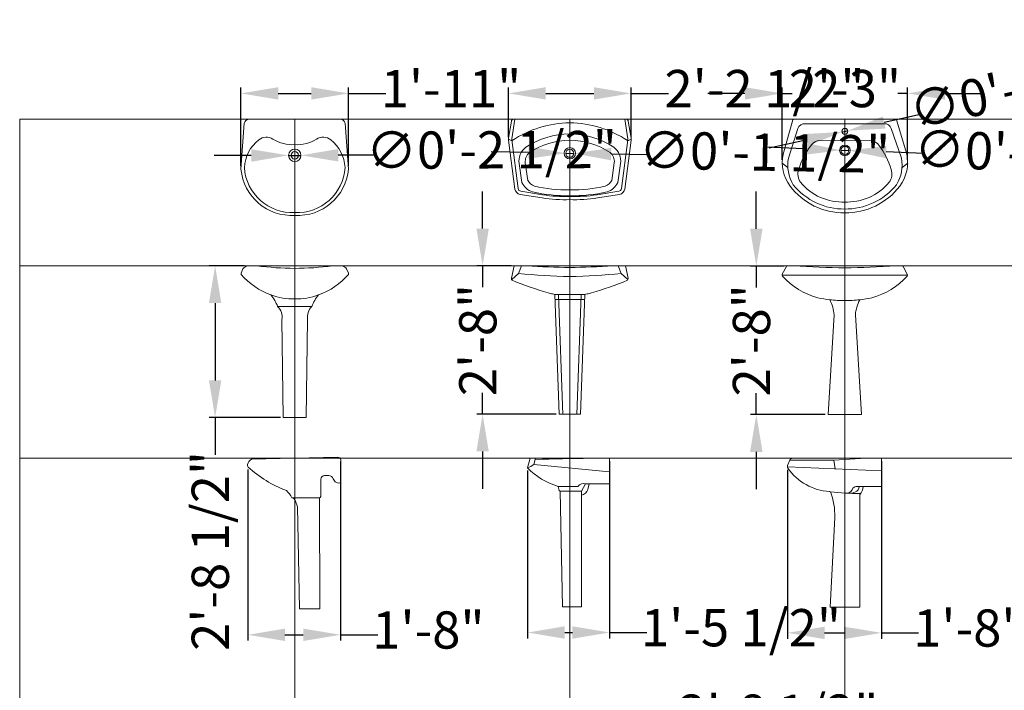
# Model space of a CAD drawing. Units: inches. Extents: x 2138 to 3265, y 2149 to 3392.
# Tile 9 of 13: x 2828 to 3040, y 3248 to 3392. Entities that reach past the tile are written whole.
import ezdxf

# ---------------------------------------------------------------- set-up
doc = ezdxf.new("R2010")
doc.units = ezdxf.units.IN
for name, color, linetype, lineweight in [('A-ANNO-DIMS', 2, 'Continuous', 18), ('A-DETL-GRID', 1, 'Continuous', 13), ('Washbasin-detail', 251, 'Continuous', 13), ('Washbasin-outline', 250, 'Continuous', 20)]:
    doc.layers.add(name, color=color, linetype=linetype, lineweight=lineweight)
doc.styles.get("Standard").update_dxf_attribs({"font": 'arial.ttf'})
doc.dimstyles.new('ISO-25', dxfattribs={"dimtxt": 8, "dimasz": 8, "dimexe": 1.25, "dimexo": 0.625, "dimtad": 0, "dimdec": 1, "dimlunit": 4, "dimtxsty": 'Standard', "dimcen": 2.5, "dimadec": 0, "dimazin": 0, "dimtfac": 1, "dimtdec": 1, "dimtmove": 0, "dimatfit": 3, "dimfxl": 1, "dimarcsym": 0})

# ---------------------------------------------------------------- blocks, each defined once
blk = doc.blocks.new('*D61')
at = {"layer": 'A-ANNO-DIMS', "color": 0, "lineweight": -2, "transparency": 16777216}
for p, q in [((2875.97, 3360.79), (2875.97, 3377.71)), ((2883.97, 3376.46), (2891.07, 3376.46)), ((2899.07, 3360.79), (2899.07, 3377.71)), ((2899.07, 3376.46), (2907.07, 3376.46))]:
    blk.add_line(p, q, dxfattribs=at)
at = {"layer": 'A-ANNO-DIMS', "color": 0, "transparency": 16777216}
for points in [[(2883.97, 3377.79), (2883.97, 3375.13), (2875.97, 3376.46)], [(2891.07, 3377.79), (2891.07, 3375.13), (2899.07, 3376.46)]]:
    blk.add_solid(points, dxfattribs=at)
at = {"layer": 'Defpoints', "color": 0, "transparency": 16777216}
for p in [(2899.07, 3376.46), (2875.97, 3360.17), (2899.07, 3360.17)]:
    blk.add_point(p, dxfattribs=at)
at = {"layer": 'A-ANNO-DIMS', "color": 0, "transparency": 16777216, "insert": (2921.06, 3376.46), "char_height": 8, "attachment_point": 5}
blk.add_mtext('1\'-11"', dxfattribs=at)
blk = doc.blocks.new('*D62')
at = {"layer": 'A-ANNO-DIMS', "color": 0, "lineweight": -2, "transparency": 16777216}
for p, q in [((2876.63, 3339.41), (2869.17, 3339.41)), ((2870.42, 3331.41), (2870.42, 3314.81)), ((2884.44, 3306.81), (2869.17, 3306.81)), ((2870.42, 3306.81), (2870.42, 3298.81))]:
    blk.add_line(p, q, dxfattribs=at)
at = {"layer": 'A-ANNO-DIMS', "color": 0, "transparency": 16777216}
for points in [[(2869.09, 3331.41), (2871.75, 3331.41), (2870.42, 3339.41)], [(2869.09, 3314.81), (2871.75, 3314.81), (2870.42, 3306.81)]]:
    blk.add_solid(points, dxfattribs=at)
at = {"layer": 'Defpoints', "color": 0, "transparency": 16777216}
for p in [(2877.25, 3339.41), (2870.42, 3306.81), (2885.06, 3306.81)]:
    blk.add_point(p, dxfattribs=at)
at = {"layer": 'A-ANNO-DIMS', "color": 0, "transparency": 16777216, "insert": (2870.42, 3278.16), "char_height": 8, "attachment_point": 5, "rotation": 90}
blk.add_mtext('2\'-8 1/2"', dxfattribs=at)
blk = doc.blocks.new('*D63')
at = {"layer": 'A-ANNO-DIMS', "color": 0, "lineweight": -2, "transparency": 16777216}
for p, q in [((2877.41, 3295.67), (2877.41, 3258.89)), ((2897.33, 3297.34), (2897.33, 3258.89)), ((2885.41, 3260.14), (2889.33, 3260.14)), ((2897.33, 3260.14), (2905.33, 3260.14))]:
    blk.add_line(p, q, dxfattribs=at)
at = {"layer": 'A-ANNO-DIMS', "color": 0, "transparency": 16777216}
for points in [[(2885.41, 3261.47), (2885.41, 3258.81), (2877.41, 3260.14)], [(2889.33, 3261.47), (2889.33, 3258.81), (2897.33, 3260.14)]]:
    blk.add_solid(points, dxfattribs=at)
at = {"layer": 'Defpoints', "color": 0, "transparency": 16777216}
for p in [(2897.33, 3297.96), (2877.41, 3296.29), (2897.33, 3260.14)]:
    blk.add_point(p, dxfattribs=at)
at = {"layer": 'A-ANNO-DIMS', "color": 0, "transparency": 16777216, "insert": (2916.21, 3260.14), "char_height": 8, "attachment_point": 5}
blk.add_mtext('1\'-8"', dxfattribs=at)
blk = doc.blocks.new('*D64')
at = {"layer": 'A-ANNO-DIMS', "color": 0, "lineweight": -2, "transparency": 16777216}
for p, q in [((2933.41, 3367.03), (2933.41, 3377.71)), ((2941.41, 3376.46), (2951.73, 3376.46)), ((2959.73, 3367.03), (2959.73, 3377.71)), ((2959.73, 3376.46), (2967.73, 3376.46))]:
    blk.add_line(p, q, dxfattribs=at)
at = {"layer": 'A-ANNO-DIMS', "color": 0, "transparency": 16777216}
for points in [[(2941.41, 3377.79), (2941.41, 3375.13), (2933.41, 3376.46)], [(2951.73, 3377.79), (2951.73, 3375.13), (2959.73, 3376.46)]]:
    blk.add_solid(points, dxfattribs=at)
at = {"layer": 'Defpoints', "color": 0, "transparency": 16777216}
for p in [(2959.73, 3376.46), (2933.41, 3366.41), (2959.73, 3366.41)]:
    blk.add_point(p, dxfattribs=at)
at = {"layer": 'A-ANNO-DIMS', "color": 0, "transparency": 16777216, "insert": (2988.38, 3376.46), "char_height": 8, "attachment_point": 5}
blk.add_mtext('2\'-2 1/2"', dxfattribs=at)
blk = doc.blocks.new('*D65')
at = {"layer": 'A-ANNO-DIMS', "color": 0, "lineweight": -2, "transparency": 16777216}
for p, q in [((2927.85, 3347.41), (2927.85, 3355.41)), ((2933.98, 3339.41), (2926.6, 3339.41)), ((2927.85, 3339.41), (2927.85, 3334.8)), ((2927.85, 3307.53), (2927.85, 3312.15)), ((2943.66, 3307.53), (2926.6, 3307.53)), ((2927.85, 3299.53), (2927.85, 3291.53))]:
    blk.add_line(p, q, dxfattribs=at)
at = {"layer": 'A-ANNO-DIMS', "color": 0, "transparency": 16777216}
for points in [[(2926.52, 3347.41), (2929.18, 3347.41), (2927.85, 3339.41)], [(2926.52, 3299.53), (2929.18, 3299.53), (2927.85, 3307.53)]]:
    blk.add_solid(points, dxfattribs=at)
at = {"layer": 'Defpoints', "color": 0, "transparency": 16777216}
for p in [(2934.6, 3339.41), (2927.85, 3307.53), (2944.29, 3307.53)]:
    blk.add_point(p, dxfattribs=at)
at = {"layer": 'A-ANNO-DIMS', "color": 0, "transparency": 16777216, "insert": (2927.85, 3323.47), "char_height": 8, "attachment_point": 5, "rotation": 90}
blk.add_mtext('2\'-8"', dxfattribs=at)
blk = doc.blocks.new('*D66')
at = {"layer": 'A-ANNO-DIMS', "color": 0, "lineweight": -2, "transparency": 16777216}
for p, q in [((2955.12, 3297.45), (2955.12, 3259.38)), ((2937.48, 3295.44), (2937.48, 3259.38)), ((2945.48, 3260.63), (2947.12, 3260.63)), ((2955.12, 3260.63), (2963.12, 3260.63))]:
    blk.add_line(p, q, dxfattribs=at)
at = {"layer": 'A-ANNO-DIMS', "color": 0, "transparency": 16777216}
for points in [[(2945.48, 3261.97), (2945.48, 3259.3), (2937.48, 3260.63)], [(2947.12, 3261.97), (2947.12, 3259.3), (2955.12, 3260.63)]]:
    blk.add_solid(points, dxfattribs=at)
at = {"layer": 'Defpoints', "color": 0, "transparency": 16777216}
for p in [(2955.12, 3298.07), (2937.48, 3296.06), (2955.12, 3260.63)]:
    blk.add_point(p, dxfattribs=at)
at = {"layer": 'A-ANNO-DIMS', "color": 0, "transparency": 16777216, "insert": (2983.32, 3260.63), "char_height": 8, "attachment_point": 5}
blk.add_mtext('1\'-5 1/2"', dxfattribs=at)
blk = doc.blocks.new('*D67')
at = {"layer": 'A-ANNO-DIMS', "color": 0, "lineweight": -2, "transparency": 16777216}
for p, q in [((2984.17, 3376.46), (2976.17, 3376.46)), ((2992.17, 3362.21), (2992.17, 3377.71)), ((2992.17, 3376.46), (2994.3, 3376.46)), ((3019.1, 3376.46), (3016.96, 3376.46)), ((3019.1, 3362.21), (3019.1, 3377.71)), ((3027.1, 3376.46), (3035.1, 3376.46))]:
    blk.add_line(p, q, dxfattribs=at)
at = {"layer": 'A-ANNO-DIMS', "color": 0, "transparency": 16777216}
for points in [[(2984.17, 3377.79), (2984.17, 3375.13), (2992.17, 3376.46)], [(3027.1, 3377.79), (3027.1, 3375.13), (3019.1, 3376.46)]]:
    blk.add_solid(points, dxfattribs=at)
at = {"layer": 'Defpoints', "color": 0, "transparency": 16777216}
for p in [(3019.1, 3376.46), (2992.17, 3361.58), (3019.1, 3361.58)]:
    blk.add_point(p, dxfattribs=at)
at = {"layer": 'A-ANNO-DIMS', "color": 0, "transparency": 16777216, "insert": (3005.63, 3376.46), "char_height": 8, "attachment_point": 5}
blk.add_mtext('2\'-3"', dxfattribs=at)
blk = doc.blocks.new('*D68')
at = {"layer": 'A-ANNO-DIMS', "color": 0, "lineweight": -2, "transparency": 16777216}
for p, q in [((2986.61, 3347.37), (2986.61, 3355.37)), ((2992.55, 3339.37), (2985.36, 3339.37)), ((2986.61, 3339.37), (2986.61, 3334.73)), ((2986.61, 3307.44), (2986.61, 3312.08)), ((3001.42, 3307.44), (2985.36, 3307.44)), ((2986.61, 3299.44), (2986.61, 3291.44))]:
    blk.add_line(p, q, dxfattribs=at)
at = {"layer": 'A-ANNO-DIMS', "color": 0, "transparency": 16777216}
for points in [[(2985.27, 3347.37), (2987.94, 3347.37), (2986.61, 3339.37)], [(2985.27, 3299.44), (2987.94, 3299.44), (2986.61, 3307.44)]]:
    blk.add_solid(points, dxfattribs=at)
at = {"layer": 'Defpoints', "color": 0, "transparency": 16777216}
for p in [(2993.18, 3339.37), (2986.61, 3307.44), (3002.05, 3307.44)]:
    blk.add_point(p, dxfattribs=at)
at = {"layer": 'A-ANNO-DIMS', "color": 0, "transparency": 16777216, "insert": (2986.61, 3323.41), "char_height": 8, "attachment_point": 5, "rotation": 90}
blk.add_mtext('2\'-8"', dxfattribs=at)
blk = doc.blocks.new('*D69')
at = {"layer": 'A-ANNO-DIMS', "color": 0, "lineweight": -2, "transparency": 16777216}
for p, q in [((2993.28, 3295.6), (2993.28, 3259.31)), ((3013.46, 3297.45), (3013.46, 3259.31)), ((3001.28, 3260.56), (3005.46, 3260.56)), ((3013.46, 3260.56), (3021.46, 3260.56))]:
    blk.add_line(p, q, dxfattribs=at)
at = {"layer": 'A-ANNO-DIMS', "color": 0, "transparency": 16777216}
for points in [[(3001.28, 3261.89), (3001.28, 3259.22), (2993.28, 3260.56)], [(3005.46, 3261.89), (3005.46, 3259.22), (3013.46, 3260.56)]]:
    blk.add_solid(points, dxfattribs=at)
at = {"layer": 'Defpoints', "color": 0, "transparency": 16777216}
for p in [(3013.46, 3298.07), (2993.28, 3296.23), (3013.46, 3260.56)]:
    blk.add_point(p, dxfattribs=at)
at = {"layer": 'A-ANNO-DIMS', "color": 0, "transparency": 16777216, "insert": (3032.34, 3260.56), "char_height": 8, "attachment_point": 5}
blk.add_mtext('1\'-8"', dxfattribs=at)
blk = doc.blocks.new('*D82')
at = {"layer": 'A-ANNO-DIMS', "color": 0, "lineweight": -2, "transparency": 16777216}
for p, q in [((2930.43, 3229.45), (2930.43, 3243.52)), ((2962.71, 3229.45), (2962.71, 3243.52)), ((2938.43, 3242.27), (2954.71, 3242.27)), ((2962.71, 3242.27), (2970.71, 3242.27))]:
    blk.add_line(p, q, dxfattribs=at)
at = {"layer": 'A-ANNO-DIMS', "color": 0, "transparency": 16777216}
for points in [[(2938.43, 3243.6), (2938.43, 3240.94), (2930.43, 3242.27)], [(2954.71, 3243.6), (2954.71, 3240.94), (2962.71, 3242.27)]]:
    blk.add_solid(points, dxfattribs=at)
at = {"layer": 'Defpoints', "color": 0, "transparency": 16777216}
for p in [(2962.71, 3242.27), (2930.43, 3228.82), (2962.71, 3228.82)]:
    blk.add_point(p, dxfattribs=at)
at = {"layer": 'A-ANNO-DIMS', "color": 0, "transparency": 16777216, "insert": (2991.36, 3242.27), "char_height": 8, "attachment_point": 5}
blk.add_mtext('2\'-8 1/2"', dxfattribs=at)
blk = doc.blocks.new('*D111')
at = {"layer": 'A-ANNO-DIMS', "color": 0, "lineweight": -2, "transparency": 16777216}
for p, q in [((2878.18, 3363.11), (2870.18, 3363.09)), ((2886.18, 3363.14), (2888.85, 3363.15)), ((2904.85, 3363.21), (2896.85, 3363.18))]:
    blk.add_line(p, q, dxfattribs=at)
at = {"layer": 'A-ANNO-DIMS', "color": 0, "transparency": 16777216}
for points in [[(2878.18, 3364.45), (2878.19, 3361.78), (2886.18, 3363.14)], [(2896.85, 3364.51), (2896.86, 3361.84), (2888.85, 3363.15)]]:
    blk.add_solid(points, dxfattribs=at)
at = {"layer": 'Defpoints', "color": 0, "transparency": 16777216}
for p in [(2886.18, 3363.14), (2888.85, 3363.15)]:
    blk.add_point(p, dxfattribs=at)
at = {"layer": 'A-ANNO-DIMS', "color": 0, "transparency": 16777216, "insert": (2929.78, 3363.29), "char_height": 8, "attachment_point": 5, "rotation": 0.1991}
blk.add_mtext('∅0\'-2 1/2"', dxfattribs=at)
blk = doc.blocks.new('*D112')
at = {"layer": 'A-ANNO-DIMS', "color": 0, "lineweight": -2, "transparency": 16777216}
for p, q in [((2937.71, 3363.75), (2929.71, 3363.9)), ((2945.71, 3363.6), (2947.44, 3363.57)), ((2963.44, 3363.27), (2955.44, 3363.42))]:
    blk.add_line(p, q, dxfattribs=at)
at = {"layer": 'A-ANNO-DIMS', "color": 0, "transparency": 16777216}
for points in [[(2937.73, 3365.08), (2937.68, 3362.42), (2945.71, 3363.6)], [(2955.46, 3364.75), (2955.41, 3362.09), (2947.44, 3363.57)]]:
    blk.add_solid(points, dxfattribs=at)
at = {"layer": 'Defpoints', "color": 0, "transparency": 16777216}
for p in [(2945.71, 3363.6), (2947.44, 3363.57)]:
    blk.add_point(p, dxfattribs=at)
at = {"layer": 'A-ANNO-DIMS', "color": 0, "transparency": 16777216, "insert": (2988.36, 3362.81), "char_height": 8, "attachment_point": 5, "rotation": 358.9373}
blk.add_mtext('∅0\'-1 1/2"', dxfattribs=at)
blk = doc.blocks.new('*D113')
at = {"layer": 'A-ANNO-DIMS', "color": 0, "lineweight": -2, "transparency": 16777216}
for p, q in [((3021.86, 3371.95), (3014.05, 3370.2)), ((3005.01, 3368.17), (3006.24, 3368.45)), ((2997.21, 3366.42), (2989.4, 3364.68))]:
    blk.add_line(p, q, dxfattribs=at)
at = {"layer": 'A-ANNO-DIMS', "color": 0, "transparency": 16777216}
for points in [[(3013.76, 3371.5), (3014.34, 3368.9), (3006.24, 3368.45)], [(2996.92, 3367.73), (2997.5, 3365.12), (3005.01, 3368.17)]]:
    blk.add_solid(points, dxfattribs=at)
at = {"layer": 'Defpoints', "color": 0, "transparency": 16777216}
for p in [(3005.01, 3368.17), (3006.24, 3368.45)]:
    blk.add_point(p, dxfattribs=at)
at = {"layer": 'A-ANNO-DIMS', "color": 0, "transparency": 16777216, "insert": (3046.18, 3377.39), "char_height": 8, "attachment_point": 5, "rotation": 12.6253}
blk.add_mtext('∅0\'-1 1/2"', dxfattribs=at)
blk = doc.blocks.new('*D114')
at = {"layer": 'A-ANNO-DIMS', "color": 0, "lineweight": -2, "transparency": 16777216}
for p, q in [((2996.77, 3364.56), (2988.77, 3364.88)), ((3004.76, 3364.25), (3006.49, 3364.18)), ((3022.48, 3363.55), (3014.49, 3363.87))]:
    blk.add_line(p, q, dxfattribs=at)
at = {"layer": 'A-ANNO-DIMS', "color": 0, "transparency": 16777216}
for points in [[(2996.82, 3365.9), (2996.72, 3363.23), (3004.76, 3364.25)], [(3014.54, 3365.2), (3014.44, 3362.54), (3006.49, 3364.18)]]:
    blk.add_solid(points, dxfattribs=at)
at = {"layer": 'Defpoints', "color": 0, "transparency": 16777216}
for p in [(3004.76, 3364.25), (3006.49, 3364.18)]:
    blk.add_point(p, dxfattribs=at)
at = {"layer": 'A-ANNO-DIMS', "color": 0, "transparency": 16777216, "insert": (3047.39, 3362.58), "char_height": 8, "attachment_point": 5, "rotation": 357.7522}
blk.add_mtext('∅0\'-1 1/2"', dxfattribs=at)
blk = doc.blocks.new('*D121')
at = {"layer": 'A-ANNO-DIMS', "color": 0, "lineweight": -2, "transparency": 16777216}
for p, q in [((2904.18, 3236.4), (2896.19, 3236.24)), ((2878.85, 3235.89), (2870.85, 3235.74)), ((2886.85, 3236.05), (2888.19, 3236.08))]:
    blk.add_line(p, q, dxfattribs=at)
at = {"layer": 'A-ANNO-DIMS', "color": 0, "transparency": 16777216}
for points in [[(2878.82, 3237.23), (2878.88, 3234.56), (2886.85, 3236.05)], [(2896.16, 3237.57), (2896.21, 3234.91), (2888.19, 3236.08)]]:
    blk.add_solid(points, dxfattribs=at)
at = {"layer": 'Defpoints', "color": 0, "transparency": 16777216}
for p in [(2886.85, 3236.05), (2888.19, 3236.08)]:
    blk.add_point(p, dxfattribs=at)
at = {"layer": 'A-ANNO-DIMS', "color": 0, "transparency": 16777216, "insert": (2937.49, 3237.06), "char_height": 8, "attachment_point": 5, "rotation": 1.1379}
blk.add_mtext('3X ∅0\'-1 1/2"', dxfattribs=at)

msp = doc.modelspace()

# ---------------------------------------------------------------- linework, layer by layer
at = {"layer": 'A-DETL-GRID'}
for p, q in [((2828.46, 3239.02), (2828.46, 3370.91)), ((2828.46, 3370.91), (3241.85, 3370.91)), ((2887.52, 3239.02), (2887.52, 3370.91)), ((2946.57, 3239.02), (2946.57, 3370.91)), ((3005.63, 3239.02), (3005.63, 3370.91)), ((2828.46, 3339.41), (3241.85, 3339.41)), ((2828.46, 3298.07), (3241.85, 3298.07))]:
    msp.add_line(p, q, dxfattribs=at)
at = {"layer": 'Washbasin-detail'}
for p, q in [((2934.8, 3370.91), (2934.1, 3366.71)), ((2958.35, 3370.91), (2959.04, 3366.71)), ((2934.1, 3366.5), (2935.47, 3356.01)), ((2959.05, 3366.5), (2957.67, 3356.01)), ((2993.37, 3360.51), (2992.16, 3361.5)), ((3017.89, 3360.51), (3019.11, 3361.5)), ((2936.05, 3355.42), (2940.74, 3354.68)), ((2957.1, 3355.42), (2952.41, 3354.68)), ((2883.84, 3330.69), (2887.52, 3330.69)), ((2891.19, 3330.69), (2887.52, 3330.69))]:
    msp.add_line(p, q, dxfattribs=at)
for points in [[(3005.63, 3369.92), (2997.12, 3369.92, 0.390337), (2995.55, 3368.9), (2993.49, 3362.55, 0.183446), (2994.53, 3356.85, 0.232242), (3005.63, 3351.62, 0.646667)], [(3005.52, 3369.92), (3014.02, 3369.92, -0.390337), (3015.59, 3368.9), (3017.77, 3362.55, -0.183446), (3016.74, 3356.85, -0.230237), (3005.52, 3351.62, -0.646667)], [(2937.36, 3339.41, 0.011502), (2946.57, 3339.06, 0.503451)], [(2955.79, 3339.41, -0.011502), (2946.57, 3339.06, -0.503451)], [(3005.63, 3338.98, -0.010807), (2994.64, 3339.41, -32.766404)], [(3005.58, 3338.98, 0.010807), (3016.56, 3339.41, 32.766404)], [(2935.54, 3337.77, 0.019244), (2946.57, 3337.09, 0.717217)], [(2957.61, 3337.77, -0.019244), (2946.57, 3337.09, -0.717217)], [(2939.17, 3298.07), (2938.82, 3296.7, -0.068261), (2937.48, 3296.06, -15.363981)], [(2939.13, 3297.8, -0.004356), (2950.9, 3298.07, 136.103409)], [(2944.05, 3292.01), (2948.31, 3292.01, -0.304727), (2949.96, 3292.6, 1.285505)], [(3008.66, 3292.01, -0.342017), (3007.87, 3290.83, -0.117748), (3006.61, 3290.52, 189.338615)], [(3009.57, 3292.01, -0.172288), (3008.82, 3290.25, 0.079687)], [(2886.88, 3289.57), (2892.81, 3289.57, 0.257732)]]:
    msp.add_lwpolyline(points, format="xyb", dxfattribs=at)
msp.add_lwpolyline([(2946.57, 3354.47, -0.060927), (2938.56, 3355.3, -0.198623), (2936.26, 3357.33), (2935.68, 3361.39, -0.265279), (2937.13, 3364.88, -0.145828), (2946.57, 3367.74, -0.145828), (2956.02, 3364.88, -0.265279), (2957.47, 3361.39), (2956.89, 3357.33, -0.198623), (2954.59, 3355.3, -0.060927)], format="xyb", close=True, dxfattribs=at)
for points in [[(2933.4, 3366.63), (2934.13, 3366.27)], [(2959.75, 3366.63), (2959.02, 3366.27)], [(2936.22, 3339.41), (2935.55, 3337.8), (2934.1, 3336.48)], [(2956.93, 3339.41), (2957.6, 3337.8), (2959.05, 3336.48)], [(3005.63, 3337.41), (2992.2, 3337.41)], [(3005.58, 3337.41), (3019, 3337.41)], [(2943.38, 3332.21), (2946.57, 3332.21)], [(2944.13, 3333.23), (2945.04, 3307.48)], [(2949.76, 3332.21), (2946.57, 3332.21)], [(2949.01, 3333.23), (2948.11, 3307.48)], [(2993.82, 3297.68), (3003.27, 3297.68), (3010.12, 3298.07)], [(2938.83, 3296.73), (2955.12, 3295.12)], [(2993.27, 3296.22), (3013.46, 3295.4)], [(3003.27, 3297.68), (3003.54, 3295.8)], [(2949.09, 3290.11), (2949.09, 3290.99)]]:
    msp.add_lwpolyline(points, dxfattribs=at)
for centre, radius in [((3005.63, 3368.31), 0.63), ((3005.63, 3364.22), 1.14), ((2887.52, 3363.15), 1.33), ((2887.52, 3363.15), 0.798), ((2946.57, 3363.59), 1.22), ((2946.57, 3363.59), 0.866), ((3005.63, 3364.22), 0.866)]:
    msp.add_circle(centre, radius, dxfattribs=at)
for centre, radius, start, end in [((2946.67, 3347.68), 22.44, 90.2484, 123.8167), ((2946.48, 3347.68), 22.44, 56.1833, 89.7516), ((2934.78, 3366.59), 0.685, 170.112, 187.4069), ((2958.37, 3366.59), 0.685, 352.5931, 9.888), ((2936.15, 3356.1), 0.685, 187.4069, 260.9868), ((2956.99, 3356.1), 0.685, 279.0132, 352.5931), ((2945.37, 3383.35), 29.05, 260.831, 272.3738), ((2947.77, 3383.44), 29.14, 267.63, 279.154), ((2887.87, 3405.24), 66.37, 262.663, 269.6975), ((2887.17, 3405.24), 66.37, 270.3025, 277.337)]:
    msp.add_arc(centre, radius, start, end, dxfattribs=at)
at = {"layer": 'Washbasin-outline'}
for p, q in [((2992.19, 3337.59), (2993.06, 3339.24)), ((2993.34, 3339.41), (3005.63, 3339.41)), ((3017.86, 3339.41), (3005.58, 3339.41)), ((3019.01, 3337.59), (3018.15, 3339.24)), ((2885.06, 3306.81), (2884.76, 3327.86)), ((2889.97, 3306.81), (2890.28, 3327.86)), ((2885.06, 3306.81), (2887.52, 3306.81)), ((2889.97, 3306.81), (2887.52, 3306.81)), ((2897.41, 3292.88), (2897.41, 3297.76)), ((2993.32, 3296.54), (2993.81, 3297.69)), ((2994.39, 3298.07), (3013.46, 3298.07)), ((3008.82, 3290.25), (3008.82, 3290.52)), ((3008.82, 3266.11), (3008.82, 3290.25)), ((2888.5, 3265.69), (2892.88, 3265.69))]:
    msp.add_line(p, q, dxfattribs=at)
for points in [[(2887.52, 3350.25, 0.403486), (2899.07, 3360.17), (2898.37, 3370.07, 0.28965), (2897.36, 3370.91), (2887.52, 3370.91), (2877.68, 3370.91, 0.28965), (2876.66, 3370.07), (2875.97, 3360.17, 0.403486)], [(2887.52, 3365.45, 0.15774), (2892.2, 3366.66, -0.319092), (2895.23, 3366.5, -0.21437), (2898.32, 3360.54, -0.410827), (2887.52, 3350.86, -0.410827), (2876.71, 3360.54, -0.21437), (2879.8, 3366.5, -0.319092), (2882.83, 3366.66, 0.15774)], [(2946.57, 3355.74, -0.060333), (2938.96, 3356.51, -0.170001), (2937.57, 3357.75), (2937.02, 3361.57, -0.259072), (2937.92, 3363.77, -0.144845), (2946.57, 3366.38, -0.144845), (2955.22, 3363.77, -0.259072), (2956.12, 3361.57), (2955.57, 3357.75, -0.170001), (2954.19, 3356.51, -0.060333)]]:
    msp.add_lwpolyline(points, format="xyb", close=True, dxfattribs=at)
for points in [[(2946.57, 3370.91), (2934.52, 3370.91, 0.364524), (2934.02, 3370.49), (2933.42, 3366.82, 0.075607), (2933.41, 3366.41), (2934.79, 3355.92, 0.332558), (2935.94, 3354.74), (2940.63, 3353.99, 0.050613), (2946.57, 3353.64, 0.488554)], [(2946.57, 3370.91), (2958.62, 3370.91, -0.364524), (2959.13, 3370.49), (2959.73, 3366.82, -0.075607), (2959.73, 3366.41), (2958.36, 3355.92, -0.332558), (2957.21, 3354.74), (2952.52, 3353.99, -0.050613), (2946.57, 3353.64, -0.488554)], [(3005.63, 3370.91), (2994.64, 3370.91, 0.349334), (2994.45, 3370.76), (2992.34, 3363.39, 0.210862), (2993.85, 3356.53, 0.238221), (3005.59, 3350.79, -0.006376)], [(3005.52, 3370.91), (3016.5, 3370.91, -0.349334), (3016.69, 3370.76), (3018.92, 3363.39, -0.210862), (3017.42, 3356.53, -0.236938), (3005.59, 3350.79, 0.006376)], [(3005.63, 3366.34), (2999.67, 3366.24, 0.204561), (2998.27, 3365.12, 0.107345), (2995.72, 3360.11, 0.24654), (2996.1, 3357.37, 0.234802), (3005.67, 3353.11, 0.791678)], [(3005.52, 3366.34), (3011.48, 3366.24, -0.218686), (3012.88, 3365.32, -0.103144), (3015.54, 3360.11, -0.24654), (3015.16, 3357.37, -0.232404), (3005.48, 3353.11, -0.791678)], [(2887.52, 3339.41), (2877.25, 3339.41, 0.168235), (2876.39, 3338.76), (2876.01, 3337.81), (2876.01, 3337.58, 0.131883), (2882.4, 3333.16, -0.027266)], [(2887.52, 3339.41), (2897.78, 3339.41, -0.168235), (2898.64, 3338.76), (2899.03, 3337.81), (2899.03, 3337.58, -0.131883), (2892.64, 3333.16, 0.027266)], [(2946.57, 3339.41), (2934.6, 3339.41), (2934.05, 3336.74, 0.20422), (2934.21, 3336.3, 0.03069), (2941.93, 3333.62, 0.65507)], [(2946.57, 3339.41), (2958.54, 3339.41), (2959.09, 3336.74, -0.20422), (2958.94, 3336.3, -0.03069), (2951.22, 3333.62, -0.65507)], [(2941.93, 3333.62, 0.001686), (2942.36, 3333.5, 0.65507)], [(2951.22, 3333.62, -0.001686), (2950.79, 3333.5, -0.65507)], [(2884.76, 3327.86, 0.245357), (2883.84, 3330.69, 0.083504), (2882.4, 3333.16, -4.704261)], [(2882.4, 3333.16, 0.08736), (2887.52, 3332.29, -0.027266)], [(2892.64, 3333.16, -0.08736), (2887.52, 3332.29, 0.027266)], [(2890.28, 3327.86, -0.245357), (2891.19, 3330.69, -0.083504), (2892.64, 3333.16, 4.704261)], [(2942.36, 3333.5, 0.003989), (2943.39, 3333.23, 0.65507)], [(2950.79, 3333.5, -0.003989), (2949.76, 3333.23, -0.65507)], [(3005.63, 3307.44), (3002.05, 3307.44), (3003.34, 3328.86, 0.094609), (3002.37, 3332.13, -1.525098)], [(3005.58, 3307.44), (3009.16, 3307.44), (3007.87, 3328.86, -0.094609), (3008.83, 3332.13, 1.525098)], [(2897.41, 3297.76, 0.347203), (2896.79, 3298.29), (2878.24, 3297.86, 0.195931), (2877.37, 3296.72, 0.256358), (2877.5, 3296.17, 0.096836), (2885.72, 3291.16, -0.091747), (2886.88, 3289.57, -0.251735), (2887.47, 3289.23, -0.085998), (2888.1, 3287.61), (2888.5, 3265.69)], [(2950.75, 3292.6), (2955.12, 3292.6), (2955.12, 3298.07), (2938.03, 3298.07), (2937.48, 3295.99, 0.123106), (2944.05, 3292.01), (2944.29, 3291.15, 0.236068), (2944.53, 3290.99, 0.351494)], [(3013.46, 3298.04), (3013.46, 3292.01), (3009.57, 3292.01, 0.240306)], [(2892.81, 3289.57, 0.257732), (2893.11, 3289.85), (2893.11, 3293.55, -0.398378), (2893.89, 3294.35), (2894.86, 3294.35, -0.237042), (2895.77, 3293.67, 0.1769), (2896.45, 3292.86, 0.278116), (2897.41, 3292.88, 3.717929)], [(2950.75, 3292.6), (2950.47, 3291.38, -0.215415), (2949.09, 3290.11)], [(3009.57, 3292.01), (3008.31, 3292.01, 0.240306), (3007.36, 3291.62, -0.219906), (3006.22, 3290.55, 6.2607)], [(3008.82, 3266.11), (3002.44, 3266.11), (3003.45, 3285.36, 0.103398), (3002.51, 3290.88, 5.161723)]]:
    msp.add_lwpolyline(points, format="xyb", dxfattribs=at)
for points in [[(2946.57, 3307.53), (2944.29, 3307.53), (2943.34, 3333.23)], [(2943.34, 3333.23), (2946.57, 3333.23)], [(2946.57, 3307.53), (2948.86, 3307.53), (2949.8, 3333.23), (2949.76, 3333.23)], [(2949.76, 3333.23), (2946.57, 3333.23)], [(2949.09, 3290.99), (2949.96, 3292.6), (2950.75, 3292.6)], [(2892.88, 3265.69), (2892.81, 3289.57)], [(2944.53, 3290.99), (2945, 3266.18)], [(2949.09, 3290.99), (2944.53, 3290.99)], [(2945, 3266.18), (2949.09, 3266.18), (2949.09, 3290.11)]]:
    msp.add_lwpolyline(points, dxfattribs=at)
for centre, radius, start, end in [((2993.34, 3339.09), 0.325, 90, 152.4267), ((3017.86, 3339.09), 0.325, 27.5733, 90), ((2992.48, 3337.44), 0.325, 152.4267, 221.363), ((3003.71, 3347.32), 15.28, 221.363, 255.1139), ((3007.5, 3347.32), 15.28, 284.8861, 318.637), ((3018.72, 3337.44), 0.325, 318.637, 27.5733), ((3005.81, 3361.5), 29.57, 258.2458, 263.3339), ((3005.81, 3361.5), 29.57, 258.2458, 263.3339), ((3005.81, 3361.5), 29.57, 263.3339, 269.6059), ((3005.4, 3361.5), 29.57, 270.3941, 276.6661), ((3005.4, 3361.5), 29.57, 276.6661, 281.7542), ((2994.39, 3297.44), 0.63, 90, 156.9487), ((2993.9, 3296.29), 0.63, 156.9487, 215.1468), ((3003.12, 3302.78), 11.9, 215.1468, 266.1673), ((3008.09, 3332.37), 41.86, 262.0734, 262.3523), ((3008.09, 3332.37), 41.86, 262.3523, 270.9902)]:
    msp.add_arc(centre, radius, start, end, dxfattribs=at)

# ---------------------------------------------------------------- dimensions: what is measured, and where the dimension line sits
at = {"layer": 'A-ANNO-DIMS'}
for p1, p2, picture, middle in [((3005.01, 3368.17), (3006.24, 3368.45), '*D113', (3046.18, 3377.39)), ((2945.71, 3363.6), (2947.44, 3363.57), '*D112', (2988.36, 3362.81)), ((3004.76, 3364.25), (3006.49, 3364.18), '*D114', (3047.39, 3362.58))]:
    dim = msp.add_diameter_dim_2p(p1=p1, p2=p2, dimstyle='ISO-25', override={"dimdec": 1, "dimlfac": 1, "dimrnd": 0, "dimzin": 1, "dimdsep": 46, "dimlunit": 4, "dimfrac": 2}, dxfattribs=at)
    dim.commit()
    dim.dimension.update_dxf_attribs({"geometry": picture, "text_midpoint": middle})
for base, p1, p2, picture, middle in [((2959.73, 3376.46), (2933.41, 3366.41), (2959.73, 3366.41), '*D64', (2988.38, 3376.46)), ((2899.07, 3376.46), (2875.97, 3360.17), (2899.07, 3360.17), '*D61', (2921.06, 3376.46)), ((3019.1, 3376.46), (2992.17, 3361.58), (3019.1, 3361.58), '*D67', (3005.63, 3376.46)), ((2897.33, 3260.14), (2877.41, 3296.29), (2897.33, 3297.96), '*D63', (2916.21, 3260.14)), ((2955.12, 3260.63), (2937.48, 3296.06), (2955.12, 3298.07), '*D66', (2983.32, 3260.63)), ((3013.46, 3260.56), (2993.28, 3296.23), (3013.46, 3298.07), '*D69', (3032.34, 3260.56)), ((2962.71, 3242.27), (2930.43, 3228.82), (2962.71, 3228.82), '*D82', (2991.36, 3242.27))]:
    dim = msp.add_linear_dim(base=base, p1=p1, p2=p2, dimstyle='ISO-25', override={"dimdec": 1, "dimlfac": 1, "dimrnd": 0, "dimzin": 1, "dimdsep": 46, "dimlunit": 4, "dimfrac": 2}, dxfattribs=at)
    dim.commit()
    dim.dimension.update_dxf_attribs({"geometry": picture, "text_midpoint": middle})
dim = msp.add_diameter_dim_2p(p1=(2886.18, 3363.14), p2=(2888.85, 3363.15), dimstyle='ISO-25', override={"dimdec": 1, "dimlfac": 1, "dimrnd": 0, "dimzin": 1, "dimdsep": 46, "dimlunit": 4, "dimfrac": 2}, dxfattribs=at)
dim.commit()
dim.dimension.update_dxf_attribs({"geometry": '*D111', "text_midpoint": (2929.78, 3363.29), "dimtype": 163})
for base, p1, p2, picture, middle in [((2927.85, 3307.53), (2934.6, 3339.41), (2944.29, 3307.53), '*D65', (2927.85, 3323.47)), ((2986.61, 3307.44), (2993.18, 3339.37), (3002.05, 3307.44), '*D68', (2986.61, 3323.41)), ((2870.42, 3306.81), (2877.25, 3339.41), (2885.06, 3306.81), '*D62', (2870.42, 3278.16))]:
    dim = msp.add_linear_dim(base=base, p1=p1, p2=p2, angle=90, dimstyle='ISO-25', override={"dimdec": 1, "dimlfac": 1, "dimrnd": 0, "dimzin": 1, "dimdsep": 46, "dimlunit": 4, "dimfrac": 2}, dxfattribs=at)
    dim.commit()
    dim.dimension.update_dxf_attribs({"geometry": picture, "text_midpoint": middle})
dim = msp.add_diameter_dim_2p(p1=(2886.85, 3236.05), p2=(2888.19, 3236.08), text='3X <>', dimstyle='ISO-25', override={"dimdec": 1, "dimlfac": 1, "dimrnd": 0, "dimzin": 1, "dimdsep": 46, "dimlunit": 4, "dimfrac": 2}, dxfattribs=at)
dim.commit()
dim.dimension.update_dxf_attribs({"geometry": '*D121', "text_midpoint": (2937.49, 3237.06), "dimtype": 163})

doc.saveas('drawing.dxf')
